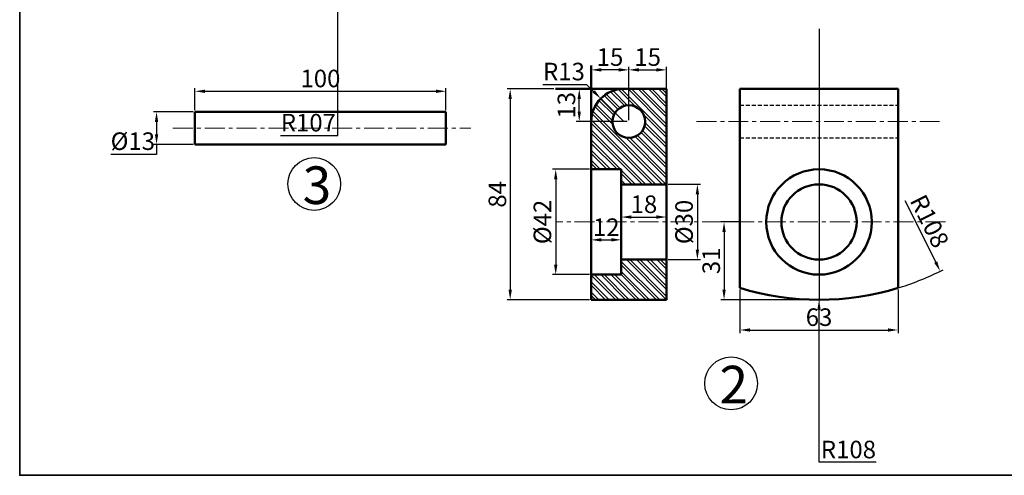
# Model space of a CAD drawing. Units: millimetres. Extents: x -108 to 732, y -172 to 297.
# Tile 1 of 4: x -108 to 284, y -172 to 9. Entities that reach past the tile are written whole.
import ezdxf

# ---------------------------------------------------------------- set-up
doc = ezdxf.new("R2010")
doc.units = ezdxf.units.MM
doc.header["$LTSCALE"] = 0.5
doc.linetypes.add('CENTER', pattern=[50.8, 31.75, -6.35, 6.35, -6.35])
doc.linetypes.add('HIDDEN', pattern=[9.525, 6.35, -3.175])
for name, color, linetype, lineweight in [('M-CNTR', 1, 'CENTER', 18), ('M-DIMS', 2, 'Continuous', 25), ('M-HATC', 8, 'Continuous', 18), ('M-HIDN', 6, 'HIDDEN', 25), ('M-OUTL', 7, 'Continuous', 50), ('M-SYMB', 3, 'Continuous', 25), ('M-TEXT', 3, 'Continuous', 25), ('M-TTLB', 7, 'Continuous', 35)]:
    doc.layers.add(name, color=color, linetype=linetype, lineweight=lineweight)
doc.styles.get("Standard").update_dxf_attribs({"font": 'arial.ttf'})
doc.dimstyles.new('ISO-25', dxfattribs={"dimtxt": 7, "dimasz": 4, "dimexe": 1.25, "dimexo": 0.625, "dimtad": 1, "dimtoh": 1, "dimtxsty": 'Standard', "dimcen": 2.5, "dimadec": 0, "dimazin": 0, "dimtfac": 1, "dimtmove": 0, "dimatfit": 3, "dimfxl": 1, "dimarcsym": 0})

# ---------------------------------------------------------------- blocks, each defined once
blk = doc.blocks.new('*D20')
at = {"layer": 'Defpoints', "color": 0, "ltscale": 0.5, "transparency": 16777216}
for p in [(-38.57, -27.57), (-53.83, -40.57), (-38.57, -40.57)]:
    blk.add_point(p, dxfattribs=at)
at = {"layer": 'M-DIMS', "color": 0, "lineweight": -2, "ltscale": 0.5, "transparency": 16777216}
for p, q in [((-39.2, -27.57), (-55.08, -27.57)), ((-53.83, -31.57), (-53.83, -36.57)), ((-39.2, -40.57), (-55.08, -40.57)), ((-53.83, -40.57), (-53.83, -44.57)), ((-53.83, -44.57), (-72.1, -44.57))]:
    blk.add_line(p, q, dxfattribs=at)
at = {"layer": 'M-DIMS', "color": 0, "ltscale": 0.5, "transparency": 16777216}
for points in [[(-54.5, -31.57), (-53.17, -31.57), (-53.83, -27.57)], [(-54.5, -36.57), (-53.17, -36.57), (-53.83, -40.57)]]:
    blk.add_solid(points, dxfattribs=at)
at = {"layer": 'M-DIMS', "color": 0, "ltscale": 0.5, "transparency": 16777216, "insert": (-63.28, -40.18), "char_height": 7, "attachment_point": 5}
blk.add_mtext('%%C13', dxfattribs=at)
blk = doc.blocks.new('*D21')
at = {"layer": 'Defpoints', "color": 0, "ltscale": 0.5, "transparency": 16777216}
for p in [(61.43, -19.38), (-38.57, -27.57), (61.43, -27.57)]:
    blk.add_point(p, dxfattribs=at)
at = {"layer": 'M-DIMS', "color": 0, "lineweight": -2, "ltscale": 0.5, "transparency": 16777216}
for p, q in [((-38.57, -26.95), (-38.57, -18.13)), ((-34.57, -19.38), (57.43, -19.38)), ((61.43, -26.95), (61.43, -18.13))]:
    blk.add_line(p, q, dxfattribs=at)
at = {"layer": 'M-DIMS', "color": 0, "ltscale": 0.5, "transparency": 16777216}
for points in [[(-34.57, -18.72), (-34.57, -20.05), (-38.57, -19.38)], [(57.43, -18.72), (57.43, -20.05), (61.43, -19.38)]]:
    blk.add_solid(points, dxfattribs=at)
at = {"layer": 'M-DIMS', "color": 0, "ltscale": 0.5, "transparency": 16777216, "insert": (11.43, -15.19), "char_height": 7, "attachment_point": 5}
blk.add_mtext('100', dxfattribs=at)
blk = doc.blocks.new('*D23')
at = {"layer": 'Defpoints', "color": 0, "ltscale": 0.5, "transparency": 16777216}
for p in [(149.26, -10.85), (134.26, -31.47), (149.26, -31.47)]:
    blk.add_point(p, dxfattribs=at)
at = {"layer": 'M-DIMS', "color": 0, "lineweight": -2, "ltscale": 0.5, "transparency": 16777216}
for p, q in [((134.26, -30.85), (134.26, -9.6)), ((138.26, -10.85), (145.26, -10.85)), ((149.26, -30.85), (149.26, -9.6))]:
    blk.add_line(p, q, dxfattribs=at)
at = {"layer": 'M-DIMS', "color": 0, "ltscale": 0.5, "transparency": 16777216}
for points in [[(138.26, -10.18), (138.26, -11.51), (134.26, -10.85)], [(145.26, -10.18), (145.26, -11.51), (149.26, -10.85)]]:
    blk.add_solid(points, dxfattribs=at)
at = {"layer": 'M-DIMS', "color": 0, "ltscale": 0.5, "transparency": 16777216, "insert": (141.76, -6.65), "char_height": 7, "attachment_point": 5}
blk.add_mtext('15', dxfattribs=at)
blk = doc.blocks.new('*D24')
at = {"layer": 'Defpoints', "color": 0, "ltscale": 0.5, "transparency": 16777216}
for p in [(119.26, -10.85), (119.26, -31.47), (134.26, -31.47)]:
    blk.add_point(p, dxfattribs=at)
at = {"layer": 'M-DIMS', "color": 0, "lineweight": -2, "ltscale": 0.5, "transparency": 16777216}
for p, q in [((119.26, -30.85), (119.26, -9.6)), ((130.26, -10.85), (123.26, -10.85)), ((134.26, -30.85), (134.26, -9.6))]:
    blk.add_line(p, q, dxfattribs=at)
at = {"layer": 'M-DIMS', "color": 0, "ltscale": 0.5, "transparency": 16777216}
for points in [[(123.26, -10.18), (123.26, -11.51), (119.26, -10.85)], [(130.26, -10.18), (130.26, -11.51), (134.26, -10.85)]]:
    blk.add_solid(points, dxfattribs=at)
at = {"layer": 'M-DIMS', "color": 0, "ltscale": 0.5, "transparency": 16777216, "insert": (126.76, -6.65), "char_height": 7, "attachment_point": 5}
blk.add_mtext('15', dxfattribs=at)
blk = doc.blocks.new('*D25')
at = {"layer": 'Defpoints', "color": 0, "ltscale": 0.5, "transparency": 16777216}
for p in [(114.51, -18.47), (134.26, -18.47), (134.26, -31.47)]:
    blk.add_point(p, dxfattribs=at)
at = {"layer": 'M-DIMS', "color": 0, "lineweight": -2, "ltscale": 0.5, "transparency": 16777216}
for p, q in [((133.64, -18.47), (113.26, -18.47)), ((114.51, -27.47), (114.51, -22.47)), ((133.64, -31.47), (113.26, -31.47))]:
    blk.add_line(p, q, dxfattribs=at)
at = {"layer": 'M-DIMS', "color": 0, "ltscale": 0.5, "transparency": 16777216}
for points in [[(113.84, -22.47), (115.17, -22.47), (114.51, -18.47)], [(113.84, -27.47), (115.17, -27.47), (114.51, -31.47)]]:
    blk.add_solid(points, dxfattribs=at)
at = {"layer": 'M-DIMS', "color": 0, "ltscale": 0.5, "transparency": 16777216, "insert": (110.31, -24.97), "char_height": 7, "attachment_point": 5, "rotation": 90}
blk.add_mtext('13', dxfattribs=at)
blk = doc.blocks.new('*D26')
at = {"layer": 'Defpoints', "color": 0, "ltscale": 0.5, "transparency": 16777216}
for p in [(105.02, -18.47), (87, -102.47), (119.26, -102.47)]:
    blk.add_point(p, dxfattribs=at)
at = {"layer": 'M-DIMS', "color": 0, "lineweight": -2, "ltscale": 0.5, "transparency": 16777216}
for p, q in [((104.4, -18.47), (85.75, -18.47)), ((87, -22.47), (87, -98.47)), ((118.64, -102.47), (85.75, -102.47))]:
    blk.add_line(p, q, dxfattribs=at)
at = {"layer": 'M-DIMS', "color": 0, "ltscale": 0.5, "transparency": 16777216}
for points in [[(86.33, -22.47), (87.67, -22.47), (87, -18.47)], [(86.33, -98.47), (87.67, -98.47), (87, -102.47)]]:
    blk.add_solid(points, dxfattribs=at)
at = {"layer": 'M-DIMS', "color": 0, "ltscale": 0.5, "transparency": 16777216, "insert": (82.8, -60.47), "char_height": 7, "attachment_point": 5, "rotation": 90}
blk.add_mtext('84', dxfattribs=at)
blk = doc.blocks.new('*D27')
at = {"layer": 'Defpoints', "color": 0, "ltscale": 0.5, "transparency": 16777216}
for p in [(119.26, -50.47), (105.14, -92.47), (119.26, -92.47)]:
    blk.add_point(p, dxfattribs=at)
at = {"layer": 'M-DIMS', "color": 0, "lineweight": -2, "ltscale": 0.5, "transparency": 16777216}
for p, q in [((118.64, -50.47), (103.89, -50.47)), ((105.14, -54.47), (105.14, -88.47)), ((118.64, -92.47), (103.89, -92.47))]:
    blk.add_line(p, q, dxfattribs=at)
at = {"layer": 'M-DIMS', "color": 0, "ltscale": 0.5, "transparency": 16777216}
for points in [[(104.47, -54.47), (105.8, -54.47), (105.14, -50.47)], [(104.47, -88.47), (105.8, -88.47), (105.14, -92.47)]]:
    blk.add_solid(points, dxfattribs=at)
at = {"layer": 'M-DIMS', "color": 0, "ltscale": 0.5, "transparency": 16777216, "insert": (100.74, -71.47), "char_height": 7, "attachment_point": 5, "rotation": 90}
blk.add_mtext('%%C42', dxfattribs=at)
blk = doc.blocks.new('*D28')
at = {"layer": 'Defpoints', "color": 0, "ltscale": 0.5, "transparency": 16777216}
for p in [(149.26, -69.51), (131.26, -71.47), (149.26, -71.47)]:
    blk.add_point(p, dxfattribs=at)
at = {"layer": 'M-DIMS', "color": 0, "lineweight": -2, "ltscale": 0.5, "transparency": 16777216}
for p, q in [((131.26, -70.85), (131.26, -68.26)), ((135.26, -69.51), (145.26, -69.51)), ((149.26, -70.85), (149.26, -68.26))]:
    blk.add_line(p, q, dxfattribs=at)
at = {"layer": 'M-DIMS', "color": 0, "ltscale": 0.5, "transparency": 16777216}
for points in [[(135.26, -68.84), (135.26, -70.18), (131.26, -69.51)], [(145.26, -68.84), (145.26, -70.18), (149.26, -69.51)]]:
    blk.add_solid(points, dxfattribs=at)
at = {"layer": 'M-DIMS', "color": 0, "ltscale": 0.5, "transparency": 16777216, "insert": (140.26, -65.31), "char_height": 7, "attachment_point": 5}
blk.add_mtext('18', dxfattribs=at)
blk = doc.blocks.new('*D29')
at = {"layer": 'Defpoints', "color": 0, "ltscale": 0.5, "transparency": 16777216}
for p in [(119.26, -71.47), (131.26, -71.47), (131.26, -78.6)]:
    blk.add_point(p, dxfattribs=at)
at = {"layer": 'M-DIMS', "color": 0, "lineweight": -2, "ltscale": 0.5, "transparency": 16777216}
for p, q in [((119.26, -72.1), (119.26, -79.85)), ((131.26, -72.1), (131.26, -79.85)), ((123.26, -78.6), (127.26, -78.6))]:
    blk.add_line(p, q, dxfattribs=at)
at = {"layer": 'M-DIMS', "color": 0, "ltscale": 0.5, "transparency": 16777216}
for points in [[(123.26, -77.93), (123.26, -79.27), (119.26, -78.6)], [(127.26, -77.93), (127.26, -79.27), (131.26, -78.6)]]:
    blk.add_solid(points, dxfattribs=at)
at = {"layer": 'M-DIMS', "color": 0, "ltscale": 0.5, "transparency": 16777216, "insert": (125.26, -74.46), "char_height": 7, "attachment_point": 5}
blk.add_mtext('12', dxfattribs=at)
blk = doc.blocks.new('*D30')
at = {"layer": 'Defpoints', "color": 0, "ltscale": 0.5, "transparency": 16777216}
for p in [(149.26, -56.47), (149.26, -86.47), (161.55, -86.47)]:
    blk.add_point(p, dxfattribs=at)
at = {"layer": 'M-DIMS', "color": 0, "lineweight": -2, "ltscale": 0.5, "transparency": 16777216}
for p, q in [((149.89, -56.47), (162.8, -56.47)), ((161.55, -60.47), (161.55, -82.47)), ((149.89, -86.47), (162.8, -86.47))]:
    blk.add_line(p, q, dxfattribs=at)
at = {"layer": 'M-DIMS', "color": 0, "ltscale": 0.5, "transparency": 16777216}
for points in [[(160.89, -60.47), (162.22, -60.47), (161.55, -56.47)], [(160.89, -82.47), (162.22, -82.47), (161.55, -86.47)]]:
    blk.add_solid(points, dxfattribs=at)
at = {"layer": 'M-DIMS', "color": 0, "ltscale": 0.5, "transparency": 16777216, "insert": (157.16, -71.47), "char_height": 7, "attachment_point": 5, "rotation": 90}
blk.add_mtext('%%C30', dxfattribs=at)
blk = doc.blocks.new('*D31')
at = {"layer": 'Defpoints', "color": 0, "ltscale": 0.5, "transparency": 16777216}
for p in [(210, 5.53), (258.26, -91.09)]:
    blk.add_point(p, dxfattribs=at)
at = {"layer": 'M-DIMS', "color": 0, "lineweight": -2, "ltscale": 0.5, "transparency": 16777216}
blk.add_line((244.22, -62.97), (256.48, -87.51), dxfattribs=at)
blk.add_arc((210, 5.53), 108, 287.2893, 297.2097, dxfattribs=at)
at = {"layer": 'M-DIMS', "color": 0, "ltscale": 0.5, "transparency": 16777216}
blk.add_solid([(257.07, -87.21), (255.88, -87.81), (258.26, -91.09)], dxfattribs=at)
at = {"layer": 'M-DIMS', "color": 0, "ltscale": 0.5, "transparency": 16777216, "insert": (253.21, -71.57), "char_height": 7, "attachment_point": 5, "rotation": 296.5465}
blk.add_mtext('R108', dxfattribs=at)
blk = doc.blocks.new('*D32')
at = {"layer": 'Defpoints', "color": 0, "ltscale": 0.5, "transparency": 16777216}
for p in [(178.5, -97.78), (241.5, -97.78), (241.5, -114.53)]:
    blk.add_point(p, dxfattribs=at)
at = {"layer": 'M-DIMS', "color": 0, "lineweight": -2, "ltscale": 0.5, "transparency": 16777216}
for p, q in [((178.5, -98.4), (178.5, -115.78)), ((241.5, -98.4), (241.5, -115.78)), ((182.5, -114.53), (237.5, -114.53))]:
    blk.add_line(p, q, dxfattribs=at)
at = {"layer": 'M-DIMS', "color": 0, "ltscale": 0.5, "transparency": 16777216}
for points in [[(182.5, -113.86), (182.5, -115.19), (178.5, -114.53)], [(237.5, -113.86), (237.5, -115.19), (241.5, -114.53)]]:
    blk.add_solid(points, dxfattribs=at)
at = {"layer": 'M-DIMS', "color": 0, "ltscale": 0.5, "transparency": 16777216, "insert": (210, -110.32), "char_height": 7, "attachment_point": 5}
blk.add_mtext('63', dxfattribs=at)
blk = doc.blocks.new('*D33')
at = {"layer": 'Defpoints', "color": 0, "ltscale": 0.5, "transparency": 16777216}
for p in [(178.5, -71.47), (172.17, -102.47), (209.5, -102.47)]:
    blk.add_point(p, dxfattribs=at)
at = {"layer": 'M-DIMS', "color": 0, "lineweight": -2, "ltscale": 0.5, "transparency": 16777216}
for p, q in [((177.87, -71.47), (170.92, -71.47)), ((172.17, -75.47), (172.17, -98.47)), ((208.87, -102.47), (170.92, -102.47))]:
    blk.add_line(p, q, dxfattribs=at)
at = {"layer": 'M-DIMS', "color": 0, "ltscale": 0.5, "transparency": 16777216}
for points in [[(171.51, -75.47), (172.84, -75.47), (172.17, -71.47)], [(171.51, -98.47), (172.84, -98.47), (172.17, -102.47)]]:
    blk.add_solid(points, dxfattribs=at)
at = {"layer": 'M-DIMS', "color": 0, "ltscale": 0.5, "transparency": 16777216, "insert": (167.97, -86.97), "char_height": 7, "attachment_point": 5, "rotation": 90}
blk.add_mtext('31', dxfattribs=at)
blk = doc.blocks.new('*D56')
at = {"layer": 'Defpoints', "color": 0, "ltscale": 0.5, "transparency": 16777216}
for p in [(18.34, 134.21), (18.34, 27.21)]:
    blk.add_point(p, dxfattribs=at)
at = {"layer": 'M-DIMS', "color": 0, "lineweight": -2, "ltscale": 0.5, "transparency": 16777216}
for p, q in [((18.34, 134.21), (18.34, 27.21)), ((18.34, -36.99), (18.34, 23.21)), ((-4.45, -36.99), (18.34, -36.99))]:
    blk.add_line(p, q, dxfattribs=at)
at = {"layer": 'M-DIMS', "color": 0, "ltscale": 0.5, "transparency": 16777216}
blk.add_solid([(17.67, 23.21), (19.01, 23.21), (18.34, 27.21)], dxfattribs=at)
at = {"layer": 'M-DIMS', "color": 0, "ltscale": 0.5, "transparency": 16777216, "insert": (6.63, -32.79), "char_height": 7, "attachment_point": 5}
blk.add_mtext('R107', dxfattribs=at)
blk = doc.blocks.new('*D57')
at = {"layer": 'Defpoints', "color": 0, "ltscale": 0.5, "transparency": 16777216}
for p in [(123.07, -22.28), (132.26, -31.47)]:
    blk.add_point(p, dxfattribs=at)
at = {"layer": 'M-DIMS', "color": 0, "lineweight": -2, "ltscale": 0.5, "transparency": 16777216}
for p, q in [((100.06, -16.62), (117.41, -16.62)), ((117.41, -16.62), (120.24, -19.45)), ((132.26, -31.47), (123.07, -22.28))]:
    blk.add_line(p, q, dxfattribs=at)
at = {"layer": 'M-DIMS', "color": 0, "ltscale": 0.5, "transparency": 16777216}
blk.add_solid([(120.71, -18.98), (119.77, -19.92), (123.07, -22.28)], dxfattribs=at)
at = {"layer": 'M-DIMS', "color": 0, "ltscale": 0.5, "transparency": 16777216, "insert": (108.42, -12.42), "char_height": 7, "attachment_point": 5}
blk.add_mtext('R13', dxfattribs=at)
blk = doc.blocks.new('*D58')
at = {"layer": 'Defpoints', "color": 0, "ltscale": 0.5, "transparency": 16777216}
for p in [(210, 5.53), (210, -102.47)]:
    blk.add_point(p, dxfattribs=at)
at = {"layer": 'M-DIMS', "color": 0, "lineweight": -2, "ltscale": 0.5, "transparency": 16777216}
for p, q in [((210, 5.53), (210, -102.47)), ((210, -167.27), (210, -106.47)), ((232.8, -167.27), (210, -167.27))]:
    blk.add_line(p, q, dxfattribs=at)
at = {"layer": 'M-DIMS', "color": 0, "ltscale": 0.5, "transparency": 16777216}
blk.add_solid([(210.66, -106.47), (209.33, -106.47), (210, -102.47)], dxfattribs=at)
at = {"layer": 'M-DIMS', "color": 0, "ltscale": 0.5, "transparency": 16777216, "insert": (221.71, -163.07), "char_height": 7, "attachment_point": 5}
blk.add_mtext('R108', dxfattribs=at)

msp = doc.modelspace()

# ---------------------------------------------------------------- hatches: boundary and pattern name
at = {"layer": 'M-HATC', "ltscale": 0.5}
h = msp.add_hatch(dxfattribs=at)
h.set_pattern_fill('ANSI32', color=256, scale=0.3, angle=90)
h.set_pattern_definition([(135, (-139.1026, 3e-14), (-2.020558, -2.020558), []), (135, (-139.1026, 1.347), (-2.020558, -2.020558), [])])
h.paths.add_polyline_path([(131.263, -50.473), (131.263, -56.473), (149.263, -56.473), (149.263, -18.473), (132.263, -18.473, 0.4142136), (119.263, -31.473), (119.263, -50.473)])
h.paths.add_polyline_path([(127.763, -31.473, -1), (140.763, -31.473, -1)], flags=16)
h.paths.add_polyline_path([(131.263, -86.473), (131.263, -92.473), (119.263, -92.473), (119.263, -102.473), (149.263, -102.473), (149.263, -86.473)])

# ---------------------------------------------------------------- linework, layer by layer
at = {"layer": 'M-CNTR', "ltscale": 0.5}
for p, q in [((209.997, -117.449), (209.997, -10.75)), ((-47.334, -34.073), (71.396, -34.073)), ((161.196, -31.473), (258.798, -31.473)), ((260.32, -71.473), (105.137, -71.473))]:
    msp.add_line(p, q, dxfattribs=at)
at = {"layer": 'M-HIDN', "ltscale": 0.5}
for p, q in [((178.497, -24.973), (241.497, -24.973)), ((178.497, -37.973), (241.497, -37.973))]:
    msp.add_line(p, q, dxfattribs=at)
at = {"layer": 'M-OUTL', "ltscale": 0.5}
for p, q in [((119.263, -102.473), (119.263, -9.079)), ((105.022, -18.473), (149.263, -18.473)), ((149.263, -18.473), (149.263, -102.473)), ((178.497, -18.473), (241.497, -18.473)), ((178.497, -97.777), (178.497, -18.473)), ((241.497, -18.473), (241.497, -97.777)), ((-38.573, -27.573), (61.427, -27.573)), ((-38.573, -40.573), (-38.573, -27.573)), ((61.427, -27.573), (61.427, -40.573)), ((61.427, -40.573), (-38.573, -40.573)), ((131.263, -50.473), (119.263, -50.473)), ((131.263, -92.473), (131.263, -50.473)), ((149.263, -56.473), (131.263, -56.473)), ((149.263, -86.473), (131.263, -86.473)), ((131.263, -92.473), (119.263, -92.473)), ((149.263, -102.473), (119.263, -102.473))]:
    msp.add_line(p, q, dxfattribs=at)
for centre, radius in [((134.263, -31.473), 6.5), ((209.997, -71.473), 21), ((209.997, -71.473), 15)]:
    msp.add_circle(centre, radius, dxfattribs=at)
for centre, radius, start, end in [((132.263, -31.473), 13, 90, 180), ((209.997, 5.527), 108, 253.04224, 286.95776)]:
    msp.add_arc(centre, radius, start, end, dxfattribs=at)
at = {"layer": 'M-SYMB', "ltscale": 0.5}
for centre in [(8.966, -56.334), (174.979, -135.803)]:
    msp.add_circle(centre, 10.513, dxfattribs=at)
at = {"layer": 'M-TTLB', "ltscale": 0.5}
msp.add_lwpolyline([(-108.335, 297.096), (732.37, 297.096), (732.37, -172.452), (-108.335, -172.452)], close=True, dxfattribs=at)

# ---------------------------------------------------------------- texts
at = {"layer": 'M-TEXT', "ltscale": 0.5, "char_height": 15, "attachment_point": 1}
for s, insert in [('3', (4.363, -49.325)), ('2', (170.377, -128.795))]:
    msp.add_mtext_dynamic_manual_height_columns(s, width=20, gutter_width=12.5, heights=[1.225], dxfattribs=dict(at, insert=insert))

# ---------------------------------------------------------------- dimensions: what is measured, and where the dimension line sits
at = {"layer": 'M-DIMS', "ltscale": 0.5}
for center, mpoint, override, picture, middle in [((18.34, 134.214), (18.34, 27.214), {"dimdec": 0, "dimlfac": 1, "dimrnd": 0, "dimzin": 0, "dimdsep": 46, "dimlunit": 2}, '*D56', (6.632, -36.986)), ((209.997, 5.527), (209.997, -102.473), {"dimdec": 0, "dimlfac": 1, "dimrnd": 0, "dimzin": 0, "dimdsep": 46, "dimlunit": 2}, '*D58', (221.712, -167.273)), ((209.997, 5.527), (258.265, -91.087), {"dimclrd": 0, "dimclre": 0, "dimclrt": 0}, '*D31', (249.454, -73.451))]:
    dim = msp.add_radius_dim(center=center, mpoint=mpoint, dimstyle='ISO-25', override=override, dxfattribs=at)
    dim.commit()
    dim.dimension.update_dxf_attribs({"geometry": picture, "text_midpoint": middle, "dimtype": 164})
for base, p1, p2, picture, middle in [((119.263, -10.848), (134.263, -31.473), (119.263, -31.473), '*D24', (126.763, -6.649)), ((149.263, -10.848), (134.263, -31.473), (149.263, -31.473), '*D23', (141.763, -6.649)), ((61.427, -19.384), (-38.573, -27.573), (61.427, -27.573), '*D21', (11.427, -15.185)), ((149.263, -69.511), (131.263, -71.473), (149.263, -71.473), '*D28', (140.263, -65.312)), ((131.263, -78.599), (119.263, -71.473), (131.263, -71.473), '*D29', (125.263, -74.459)), ((241.497, -114.526), (178.497, -97.777), (241.497, -97.777), '*D32', (209.997, -110.324))]:
    dim = msp.add_linear_dim(base=base, p1=p1, p2=p2, dimstyle='ISO-25', override={"dimclrd": 0, "dimclre": 0, "dimclrt": 0}, dxfattribs=at)
    dim.commit()
    dim.dimension.update_dxf_attribs({"geometry": picture, "text_midpoint": middle})
dim = msp.add_radius_dim(center=(132.263, -31.473), mpoint=(123.07, -22.281), dimstyle='ISO-25', override={"dimdec": 0, "dimlfac": 1, "dimrnd": 0, "dimzin": 0, "dimdsep": 46, "dimlunit": 2}, dxfattribs=at)
dim.commit()
dim.dimension.update_dxf_attribs({"geometry": '*D57', "text_midpoint": (108.425, -12.423)})
for base, p1, p2, picture, middle in [((87, -102.473), (105.022, -18.473), (119.263, -102.473), '*D26', (82.801, -60.473)), ((114.506, -18.473), (134.263, -31.473), (134.263, -18.473), '*D25', (110.305, -24.973)), ((172.174, -102.472), (178.497, -71.473), (209.496, -102.472), '*D33', (167.973, -86.973))]:
    dim = msp.add_linear_dim(base=base, p1=p1, p2=p2, angle=90, dimstyle='ISO-25', override={"dimclrd": 0, "dimclre": 0, "dimclrt": 0}, dxfattribs=at)
    dim.commit()
    dim.dimension.update_dxf_attribs({"geometry": picture, "text_midpoint": middle})
for base, p1, p2, picture, middle in [((-53.834, -40.573), (-38.573, -27.573), (-38.573, -40.573), '*D20', (-63.281, -40.178)), ((105.137, -92.473), (119.263, -50.473), (119.263, -92.473), '*D27', (100.742, -71.473)), ((161.552, -86.473), (149.263, -56.473), (149.263, -86.473), '*D30', (157.157, -71.473))]:
    dim = msp.add_linear_dim(base=base, p1=p1, p2=p2, angle=90, text='%%C<>', dimstyle='ISO-25', override={"dimclrd": 0, "dimclre": 0, "dimclrt": 0}, dxfattribs=at)
    dim.commit()
    dim.dimension.update_dxf_attribs({"geometry": picture, "text_midpoint": middle})

doc.saveas('drawing.dxf')
